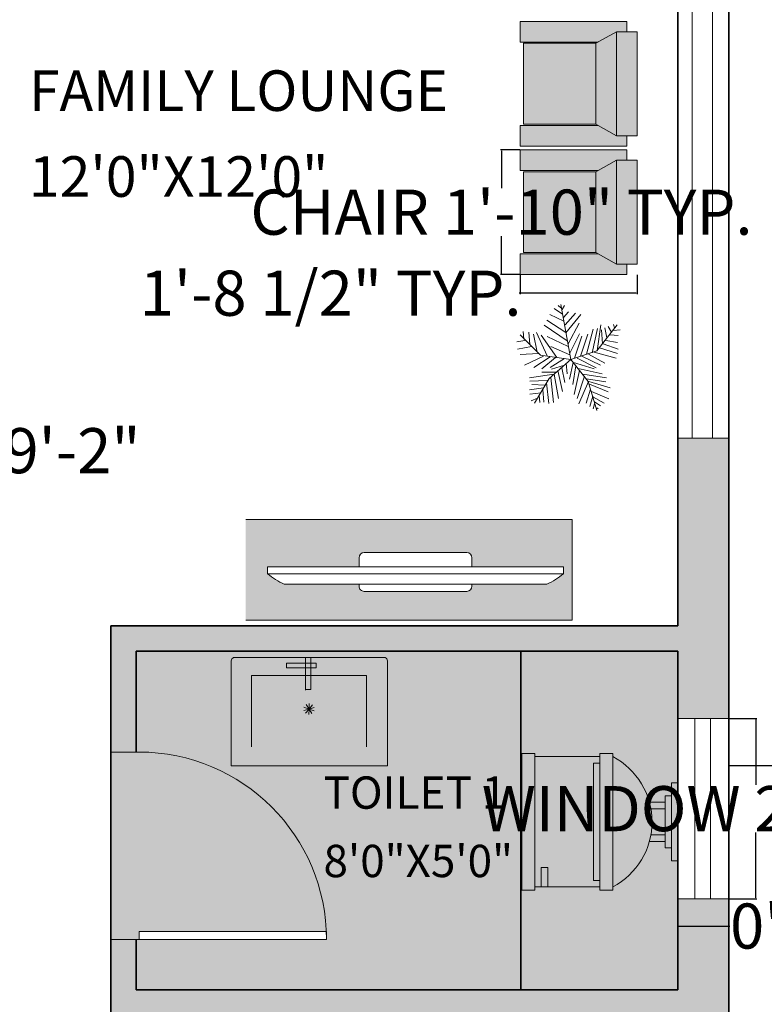
# Model space of a CAD drawing. Units: inches. Extents: x 853 to 1550, y 485 to 1596.
# Tile 10 of 18: x 1288 to 1420, y 1034 to 1208. Entities that reach past the tile are written whole.
import ezdxf

# ---------------------------------------------------------------- set-up
doc = ezdxf.new("R2010")
doc.units = ezdxf.units.IN
doc.header["$MEASUREMENT"] = 0
for name, color, linetype, lineweight in [('A-ANNO-DIMS', 2, 'Continuous', 18), ('A-AREA-IDEN', 250, 'Continuous', 18), ('A-DOOR', 4, 'Continuous', 18), ('A-FLOR-CASE', 32, 'Continuous', 25), ('A-FLOR-FIXT', 8, 'Continuous', 18), ('A-WALL-PATT', 250, 'Continuous', 13), ('furniture', 250, 'Continuous', 18), ('L-PLNT-TREE', 106, 'Continuous', 13), ('walls', 250, 'Continuous', 35), ('windows', 4, 'Continuous', 18)]:
    doc.layers.add(name, color=color, linetype=linetype, lineweight=lineweight)
for name, color, linetype, lineweight, true_color in [('A-FIXT-PATT', 9, 'Continuous', 13, 0xc7c8ca), ('A-FLOR-TILE-PATT', 141, 'Continuous', 13, 0xadddf7), ('A-FURN-PATT', 254, 'Continuous', 13, 0xfeeab9)]:
    doc.layers.add(name, color=color, linetype=linetype, lineweight=lineweight, true_color=true_color)
doc.styles.get("Standard").update_dxf_attribs({"font": 'arial.ttf'})
doc.dimstyles.get("Standard").update_dxf_attribs({"dimtxt": 8, "dimasz": 0.18, "dimexe": 0.18, "dimexo": 0.0625, "dimgap": 0.09, "dimtad": 0, "dimtih": 1, "dimtoh": 1, "dimzin": 0, "dimdsep": 46, "dimlunit": 3, "dimtxsty": 'Standard', "dimcen": 0.09, "dimadec": 0, "dimazin": 0, "dimtfac": 1, "dimtofl": 0, "dimtmove": 0, "dimatfit": 3, "dimfxl": 1, "dimtolj": 1, "dimtzin": 0, "dimarcsym": 0})

# ---------------------------------------------------------------- blocks, each defined once
blk = doc.blocks.new('*U10')
for p, q in [((0, 0), (0, -6)), ((40, 0), (40, -6))]:
    blk.add_line(p, q)
blk.add_lwpolyline([(0, 0), (0, 40), (1.75, 40), (1.75, 0)], close=True)
blk.add_arc((0, 0), 40, 0, 90)
blk = doc.blocks.new('FABRIC SOFA 1S')
at = {"layer": 'furniture'}
for p, q in [((3, 18.12), (34, 18.12)), ((3, 15.12), (3, 18.12)), ((34, 12.12), (34, 18.12)), ((0, -15.12), (0, 15.12)), ((6, 15.12), (0, 15.12)), ((6, -15.12), (6, 15.12)), ((12, 11.75), (6, 15.12)), ((11.33, 12.12), (34, 12.12)), ((6, -15.12), (12, -11.75)), ((11.33, -12.12), (34, -12.12)), ((34, -12.12), (34, -18.12)), ((6, -15.12), (0, -15.12)), ((3, -18.12), (3, -15.12)), ((3, -18.12), (34, -18.12))]:
    blk.add_line(p, q, dxfattribs=at)
blk.add_lwpolyline([(12, -11.75), (12, 11.75), (33, 11.75), (33, -11.75)], close=True, dxfattribs=at)
blk = doc.blocks.new('*U5')
for p, q in [((-10, 22), (-10, 12)), ((10, 12), (10, 22)), ((-10, 21), (-7, 21)), ((-7, 20), (-10, 20)), ((-7, 21), (-7, 20)), ((9, 13), (-9, 13)), ((-9, 13), (-9, 12)), ((9, 12), (9, 13)), ((10.5, 12), (-10.5, 12)), ((-10.5, 10), (-10.5, 12)), ((10.5, 12), (10.5, 10)), ((10.5, 10), (-10.5, 10)), ((-3, 4.4065), (-3, 2)), ((-2, 2), (-2, 4.1658)), ((2, 4.1658), (2, 2)), ((3, 2), (3, 4.4065)), ((4, 2), (-4, 2)), ((-4, 2), (-4, 1)), ((4, 1), (4, 2))]:
    blk.add_line(p, q)
for points in [[(10.5, 22), (10.5, 24), (-10.5, 24), (-10.5, 22)], [(6, 0), (6, 1), (-6, 1), (-6, 0)]]:
    blk.add_lwpolyline(points, close=True)
blk.add_arc((0, 15.3333), 11.3333, 208.0725, 331.9275)
blk = doc.blocks.new('*D20')
at = {"layer": 'A-ANNO-DIMS', "color": 0, "lineweight": -2, "transparency": 16777216}
for p, q in [((1413.94, 1090.29), (1413.94, 1075.73)), ((1437.94, 1090.29), (1437.94, 1075.73)), ((1414.12, 1075.91), (1422.1, 1075.91)), ((1437.76, 1075.91), (1429.78, 1075.91))]:
    blk.add_line(p, q, dxfattribs=at)
at = {"layer": 'A-ANNO-DIMS', "color": 0, "transparency": 16777216}
for points in [[(1414.12, 1075.94), (1414.12, 1075.88), (1413.94, 1075.91)], [(1437.76, 1075.94), (1437.76, 1075.88), (1437.94, 1075.91)]]:
    blk.add_solid(points, dxfattribs=at)
at = {"layer": 'Defpoints', "color": 0, "transparency": 16777216}
for p in [(1413.94, 1090.36), (1437.94, 1090.36), (1437.94, 1075.91)]:
    blk.add_point(p, dxfattribs=at)
at = {"layer": 'A-ANNO-DIMS', "color": 0, "transparency": 16777216, "insert": (1425.94, 1075.91), "char_height": 8, "attachment_point": 5}
blk.add_mtext("\\A1;2'", dxfattribs=at)
blk = doc.blocks.new('*U18')
for p, q in [((-8.737, 47.138), (-17.069, 52.711)), ((-10.186, 53.64), (-13.084, 55.962)), ((0, 0), (-10.5, 57)), ((-9.099, 51.782), (-6.563, 55.962)), ((-7.288, 39.707), (-21.778, 46.673)), ((-7.65, 43.423), (-2.578, 49.46)), ((-5.839, 35.992), (4.667, 48.067)), ((-5.114, 27.632), (10.463, 46.673)), ((-3.665, 19.273), (-27.574, 35.527)), ((-5.114, 28.097), (-24.676, 40.636)), ((-2.941, 16.486), (8.652, 37.85)), ((16.259, 5.805), (23.142, 31.348)), ((22.055, 7.198), (27.489, 32.277)), ((27, 9), (48, 36)), ((27.127, 9.056), (31.112, 35.992)), ((31.836, 30.883), (32.561, 16.486)), ((35.096, 32.741), (37.27, 22.524)), ((38.719, 34.134), (41.979, 28.561)), ((43.791, 29.954), (51.036, 30.883)), ((44.153, 36.456), (45.239, 32.741)), ((-31.5, 4.5), (-52.5, 25.5)), ((-48.585, 21.131), (-49.309, 29.026)), ((-43.513, 28.561), (-42.427, 15.558)), ((-38.442, 26.239), (-34.819, 7.663)), ((-35.544, 28.097), (-24.314, 3.947)), ((-14.533, 2.09), (-30.834, 25.31)), ((-24.314, 23.917), (-2.941, 13.7)), ((-1.129, 6.734), (9.014, 26.704)), ((3.942, 1.625), (11.187, 24.381)), ((10.101, 3.483), (17.708, 26.239)), ((40.53, 25.775), (48.862, 24.846)), ((-47.498, 19.737), (-55.83, 18.344)), ((-40.615, 13.7), (-55.105, 10.913)), ((-20.691, 13.7), (-1.129, 4.876)), ((29.662, 12.307), (48.137, 6.269)), ((33.285, 16.486), (48.862, 10.913)), ((36.183, 19.737), (48.137, 17.88)), ((-33.37, 6.269), (-52.207, 5.34)), ((-28.299, 3.483), (-47.86, -5.805)), ((-21.416, 3.018), (-38.079, -8.128)), ((0, 0), (-31.5, 4.5)), ((-15.982, 2.09), (-30.11, -9.521)), ((0, 0), (-22.5, -19.5)), ((-6.563, 1.161), (-21.416, -8.128)), ((0, 0), (27, 9)), ((0, 0), (18, -22.5)), ((6.478, 1.625), (26.04, -8.592)), ((11.187, 3.483), (30.749, -5.805)), ((18.07, 5.805), (35.096, -3.483)), ((24.229, 7.663), (46.688, 1.625)), ((-6.563, -5.805), (-19.967, -9.985)), ((-9.461, -8.592), (-6.201, -23.453)), ((-4.752, -3.483), (-3.665, -14.629)), ((2.493, -3.019), (-1.491, -20.202)), ((1.769, -2.555), (24.229, -9.521)), ((5.029, -6.27), (2.131, -25.775)), ((7.565, -9.056), (32.198, -14.629)), ((-17.431, -15.094), (-42.789, -18.809)), ((-22.5, -19.5), (-37.5, -45)), ((-15.257, -12.772), (-30.11, -12.772)), ((-20.691, -18.345), (-17.793, -44.352)), ((-17.069, -15.094), (-12.721, -40.172)), ((-13.446, -11.378), (-8.737, -32.741)), ((9.014, -11.378), (3.58, -35.992)), ((14.085, -16.951), (6.478, -40.172)), ((12.274, -15.094), (36.907, -18.809)), ((16.259, -19.738), (36.183, -22.989)), ((-28.299, -29.026), (-42.789, -31.348)), ((-24.314, -21.596), (-42.427, -22.06)), ((-26.849, -26.24), (-40.253, -25.775)), ((-25.038, -23.918), (-22.865, -45.281)), ((18.07, -22.524), (8.289, -45.745)), ((20.244, -30.419), (15.897, -44.816)), ((18, -22.5), (27, -52.5)), ((18.433, -22.524), (40.53, -29.026)), ((19.157, -25.311), (38.719, -33.206)), ((-30.834, -34.135), (-42.427, -35.528)), ((-34.457, -39.708), (-40.978, -42.494)), ((-32.646, -36.921), (-31.921, -44.352)), ((-29.023, -30.884), (-27.936, -43.887)), ((22.78, -37.85), (19.519, -48.532)), ((21.331, -32.741), (39.081, -40.636)), ((22.78, -38.314), (34.372, -44.816)), ((24.591, -45.745), (23.142, -50.854)), ((24.591, -43.423), (30.749, -47.603)), ((26.764, -49.925), (28.213, -50.854))]:
    blk.add_line(p, q)
blk = doc.blocks.new('BASIN-RECT-WITH-MIXER')
for p, q in [((0, 3.21), (0, 19.18)), ((0, 19.18), (27.7, 19.18)), ((27.7, 19.18), (27.7, 0.61)), ((3.57, 3.21), (3.57, 15.84)), ((24, 15.84), (24, 3.21)), ((13.79, 9.14), (12.86, 9.39)), ((13.79, 9.14), (12.89, 8.8)), ((13.79, 9.14), (13.18, 9.89)), ((13.79, 9.14), (13.26, 8.33)), ((13.79, 9.14), (13.74, 10.1)), ((13.79, 9.14), (14.31, 9.95)), ((13.79, 9.14), (14.69, 9.48)), ((13.79, 9.14), (14.39, 8.39)), ((13.79, 9.14), (13.83, 8.18)), ((13.79, 9.14), (14.72, 8.89)), ((13.18, 5.79), (13.18, 0)), ((14.12, 5.69), (13.18, 5.69)), ((14.12, 0), (14.12, 5.69)), ((0, 0.61), (0, 3.21)), ((24, 3.21), (3.57, 3.21)), ((15.05, 1.84), (9.82, 1.84)), ((9.82, 1.84), (9.82, 0.98)), ((15.05, 0.98), (15.05, 1.84)), ((27.28, 0), (0.42, 0)), ((9.82, 0.98), (11.8, 0.98)), ((11.8, 0.98), (15.05, 0.98))]:
    blk.add_line(p, q)
for centre, start, end in [((0.76, 0.68), 185.6886, 243.8456), ((26.94, 0.68), 296.1544, 354.3114)]:
    blk.add_arc(centre, 0.761, start, end)
blk = doc.blocks.new('WIN-BATH-32IN')
for p, q in [((0, 32.01), (9, 32.01)), ((0, 0), (0, 32.01)), ((0, 32.01), (3.01, 32.01)), ((3.01, 32.01), (3.01, 0)), ((5.76, 0), (5.76, 32.01)), ((9, 32.01), (9, 0)), ((9, 0), (0, 0)), ((3.01, 0), (5.76, 0))]:
    blk.add_line(p, q)
blk = doc.blocks.new('WIN-94IN')
for p, q in [((0, 94.25), (9, 94.25)), ((0, 0), (0, 94.25)), ((2.54, 94.25), (2.54, 0)), ((6.1, 0), (6.1, 94.25)), ((9, 94.25), (9, 0)), ((9, 0), (0, 0)), ((2.54, 0), (6.1, 0))]:
    blk.add_line(p, q)
blk = doc.blocks.new('PLASMA-LARGE')
at = {"layer": 'furniture'}
for p, q in [((-7.26, 0), (7.26, 0)), ((-18.61, -1), (18.61, -1)), ((-8, -1), (-8, -0.74)), ((8, -1), (8, -0.74)), ((-21, -2.5), (21, -2.5)), ((-21, -2.5), (-21, -3.5)), ((21, -2.5), (21, -3.5)), ((-21, -3.5), (21, -3.5)), ((-8, -3.5), (-8, -4.76)), ((8, -3.5), (8, -4.76)), ((-7.26, -5.5), (7.26, -5.5))]:
    blk.add_line(p, q, dxfattribs=at)
for centre, radius, start, end in [((-7.26, -0.74), 0.744, 90, 180), ((7.26, -0.74), 0.744, 0, 90), ((-13.97, -11.05), 11.07, 114.7602, 129.4175), ((13.97, -11.05), 11.07, 50.5825, 65.2398), ((-7.26, -4.76), 0.744, 180, 270), ((7.26, -4.76), 0.744, 270, 0)]:
    blk.add_arc(centre, radius, start, end, dxfattribs=at)
blk = doc.blocks.new('TV-CONSOLE')
for p, q in [((0, 0), (0, 57.83)), ((0, 57.83), (17.81, 57.83)), ((17.81, 57.83), (17.81, 0))]:
    blk.add_line(p, q)
at = {"xscale": 1.249763490704796, "yscale": 1.249763490704796, "zscale": 1.249763490704796, "rotation": 270}
blk.add_blockref('PLASMA-LARGE', (12.71, 30.08), dxfattribs=at)
blk = doc.blocks.new('*D35')
at = {"layer": 'A-ANNO-DIMS', "color": 0, "lineweight": -2, "transparency": 16777216}
for p, q in [((1376.91, 1184.98), (1373.48, 1184.98)), ((1373.66, 1184.8), (1373.66, 1178.17)), ((1373.66, 1163.07), (1373.66, 1169.71)), ((1376.91, 1162.89), (1373.48, 1162.89))]:
    blk.add_line(p, q, dxfattribs=at)
at = {"layer": 'A-ANNO-DIMS', "color": 0, "transparency": 16777216}
for points in [[(1373.63, 1184.8), (1373.69, 1184.8), (1373.66, 1184.98)], [(1373.63, 1163.07), (1373.69, 1163.07), (1373.66, 1162.89)]]:
    blk.add_solid(points, dxfattribs=at)
at = {"layer": 'Defpoints', "color": 0, "transparency": 16777216}
for p in [(1373.66, 1184.98), (1376.98, 1184.98), (1376.98, 1162.89)]:
    blk.add_point(p, dxfattribs=at)
at = {"layer": 'A-ANNO-DIMS', "color": 0, "transparency": 16777216, "insert": (1373.66, 1173.94), "char_height": 8, "attachment_point": 5}
blk.add_mtext('\\A1;CHAIR 1\'-10" TYP.', dxfattribs=at)
blk = doc.blocks.new('*D36')
at = {"layer": 'A-ANNO-DIMS', "color": 0, "lineweight": -2, "transparency": 16777216}
for p, q in [((1376.98, 1162.83), (1376.98, 1159.4)), ((1397.7, 1162.83), (1397.7, 1159.4)), ((1376.98, 1159.58), (1376.8, 1159.58)), ((1397.52, 1159.58), (1377.16, 1159.58))]:
    blk.add_line(p, q, dxfattribs=at)
at = {"layer": 'A-ANNO-DIMS', "color": 0, "transparency": 16777216}
for points in [[(1377.16, 1159.61), (1377.16, 1159.55), (1376.98, 1159.58)], [(1397.52, 1159.61), (1397.52, 1159.55), (1397.7, 1159.58)]]:
    blk.add_solid(points, dxfattribs=at)
at = {"layer": 'Defpoints', "color": 0, "transparency": 16777216}
for p in [(1376.98, 1162.89), (1397.7, 1162.89), (1376.98, 1159.58)]:
    blk.add_point(p, dxfattribs=at)
at = {"layer": 'A-ANNO-DIMS', "color": 0, "transparency": 16777216, "insert": (1343.38, 1159.58), "char_height": 8, "attachment_point": 5}
blk.add_mtext('\\A1;1\'-8 1/2" TYP.', dxfattribs=at)
blk = doc.blocks.new('*D53')
at = {"layer": 'A-ANNO-DIMS', "color": 0, "lineweight": -2, "transparency": 16777216}
for p, q in [((1414, 1084.23), (1418.92, 1084.23)), ((1418.74, 1084.05), (1418.74, 1072.46)), ((1418.74, 1052.41), (1418.74, 1064)), ((1414, 1052.23), (1418.92, 1052.23))]:
    blk.add_line(p, q, dxfattribs=at)
at = {"layer": 'A-ANNO-DIMS', "color": 0, "transparency": 16777216}
for points in [[(1418.71, 1084.05), (1418.77, 1084.05), (1418.74, 1084.23)], [(1418.71, 1052.41), (1418.77, 1052.41), (1418.74, 1052.23)]]:
    blk.add_solid(points, dxfattribs=at)
at = {"layer": 'Defpoints', "color": 0, "transparency": 16777216}
for p in [(1413.94, 1084.23), (1418.74, 1084.23), (1413.94, 1052.23)]:
    blk.add_point(p, dxfattribs=at)
at = {"layer": 'A-ANNO-DIMS', "color": 0, "transparency": 16777216, "insert": (1418.74, 1068.23), "char_height": 8, "attachment_point": 5}
blk.add_mtext('\\A1;WINDOW 2\'-8" TYP.', dxfattribs=at)
blk = doc.blocks.new('*D54')
at = {"layer": 'A-ANNO-DIMS', "color": 0, "lineweight": -2, "transparency": 16777216}
for p, q in [((1404.94, 1052.16), (1404.94, 1047.25)), ((1413.94, 1052.16), (1413.94, 1047.25)), ((1405.12, 1047.43), (1413.76, 1047.43)), ((1413.94, 1047.43), (1414.12, 1047.43))]:
    blk.add_line(p, q, dxfattribs=at)
at = {"layer": 'A-ANNO-DIMS', "color": 0, "transparency": 16777216}
for points in [[(1405.12, 1047.46), (1405.12, 1047.4), (1404.94, 1047.43)], [(1413.76, 1047.46), (1413.76, 1047.4), (1413.94, 1047.43)]]:
    blk.add_solid(points, dxfattribs=at)
at = {"layer": 'Defpoints', "color": 0, "transparency": 16777216}
for p in [(1404.94, 1052.23), (1413.94, 1052.23), (1413.94, 1047.43)]:
    blk.add_point(p, dxfattribs=at)
at = {"layer": 'A-ANNO-DIMS', "color": 0, "transparency": 16777216, "insert": (1438.59, 1047.43), "char_height": 8, "attachment_point": 5}
blk.add_mtext('\\A1;0\'-9" TYP.', dxfattribs=at)
blk = doc.blocks.new('*D67')
at = {"layer": 'A-ANNO-DIMS', "color": 0, "lineweight": -2, "transparency": 16777216}
for p, q in [((1250.4, 1186.71), (1267.03, 1186.71)), ((1266.85, 1186.53), (1266.85, 1135.89)), ((1266.85, 1076.81), (1266.85, 1127.44)), ((1250.4, 1076.63), (1267.03, 1076.63))]:
    blk.add_line(p, q, dxfattribs=at)
at = {"layer": 'A-ANNO-DIMS', "color": 0, "transparency": 16777216}
for points in [[(1266.82, 1186.53), (1266.88, 1186.53), (1266.85, 1186.71)], [(1266.82, 1076.81), (1266.88, 1076.81), (1266.85, 1076.63)]]:
    blk.add_solid(points, dxfattribs=at)
at = {"layer": 'Defpoints', "color": 0, "transparency": 16777216}
for p in [(1250.34, 1186.71), (1266.85, 1186.71), (1250.34, 1076.63)]:
    blk.add_point(p, dxfattribs=at)
at = {"layer": 'A-ANNO-DIMS', "color": 0, "transparency": 16777216, "insert": (1266.85, 1131.67), "char_height": 8, "attachment_point": 5}
blk.add_mtext('\\A1;DINING SET 9\'-2"', dxfattribs=at)

msp = doc.modelspace()

# ---------------------------------------------------------------- hatches: boundary and pattern name
at = {"layer": 'A-FIXT-PATT'}
h = msp.add_hatch(color=256, dxfattribs=at)
h.dxf.hatch_style = 1
h.paths.add_polyline_path([(1349.763, 1079.188), (1329.326, 1079.188), (1329.326, 1091.817), (1338.94, 1091.817), (1338.94, 1089.338), (1339.876, 1089.338), (1339.876, 1091.817), (1349.763, 1091.817)])
h.paths.add_polyline_path([(1341.57, 1085.885, 1), (1337.519, 1085.885, 1)], flags=16)
h.paths.add_polyline_path([(1340.507, 1085.885, 1), (1338.582, 1085.885, 1)], flags=0)
h.paths.add_polyline_path([(1339.876, 1089.338), (1338.94, 1089.338), (1338.94, 1091.817), (1339.876, 1091.817)], flags=17)
h.paths.add_polyline_path([(1339.876, 1091.817), (1338.94, 1091.817), (1338.94, 1093.187), (1339.876, 1093.187)])
h.paths.add_polyline_path([(1339.876, 1093.187), (1338.94, 1093.187), (1338.94, 1094.047), (1339.876, 1094.047)])
h.paths.add_polyline_path([(1338.94, 1093.187), (1335.575, 1093.187), (1335.575, 1094.047), (1337.557, 1094.047), (1338.94, 1094.047)])
h.paths.add_polyline_path([(1340.811, 1093.187), (1339.876, 1093.187), (1339.876, 1094.047), (1340.811, 1094.047)])
h.paths.add_polyline_path([(1339.876, 1094.047), (1338.94, 1094.047), (1338.94, 1095.025), (1339.876, 1095.025)])
h.paths.add_polyline_path([(1339.876, 1095.025), (1338.94, 1095.025), (1338.94, 1096.137), (1339.876, 1096.137)])
h = msp.add_hatch(color=256, dxfattribs=at)
h.dxf.hatch_style = 1
h.paths.add_polyline_path([(1329.326, 1079.188), (1349.763, 1079.188), (1349.763, 1091.817), (1339.876, 1091.817), (1339.876, 1093.187), (1340.811, 1093.187), (1340.811, 1094.047), (1339.876, 1094.047), (1339.876, 1095.025), (1353.033, 1095.025, -0.2593488), (1353.455, 1094.417), (1353.455, 1075.844), (1325.759, 1075.844), (1325.759, 1091.817), (1325.759, 1094.417, -0.2593488), (1326.18, 1095.025), (1338.94, 1095.025), (1338.94, 1094.047), (1337.557, 1094.047), (1335.575, 1094.047), (1335.575, 1093.187), (1338.94, 1093.187), (1338.94, 1091.817), (1329.326, 1091.817)])
h = msp.add_hatch(color=256, dxfattribs=at)
h.dxf.hatch_style = 1
h.paths.add_polyline_path([(1337.519, 1085.885, -1), (1341.57, 1085.885, -1)])
h.paths.add_polyline_path([(1340.507, 1085.885, 1), (1338.582, 1085.885, 1)], flags=16)
h = msp.add_hatch(color=256, dxfattribs=at)
h.dxf.hatch_style = 1
h.paths.add_polyline_path([(1379.551, 1077.46), (1379.551, 1054.359), (1380.706, 1054.359), (1380.706, 1057.824), (1381.861, 1057.824), (1381.861, 1054.359), (1391.102, 1054.359), (1391.102, 1055.514), (1389.947, 1055.514), (1389.947, 1076.305), (1391.102, 1076.305), (1391.102, 1077.46)])
h.paths.add_polyline_path([(1377.241, 1078.038), (1377.241, 1053.781), (1379.551, 1053.781), (1379.551, 1078.038)])
h.paths.add_polyline_path([(1391.102, 1078.038), (1391.102, 1053.781), (1393.412, 1053.781), (1393.412, 1078.038)])
h.paths.add_polyline_path([(1389.947, 1076.305), (1389.947, 1055.514), (1391.102, 1055.514), (1391.102, 1076.305)], flags=17)
h.paths.add_polyline_path([(1393.412, 1077.46), (1393.412, 1054.359, 0.6000022)])
h.paths.add_polyline_path([(1400.137, 1063.599, -0.0226287), (1399.876, 1062.444), (1402.653, 1062.444), (1402.653, 1063.599)])
h.paths.add_polyline_path([(1399.876, 1069.375, -0.0226287), (1400.137, 1068.22), (1402.653, 1068.22), (1402.653, 1069.375)])
h.paths.add_polyline_path([(1402.653, 1070.53), (1402.653, 1061.289), (1403.808, 1061.289), (1403.808, 1070.53)])
h.paths.add_polyline_path([(1403.808, 1072.84), (1403.808, 1058.979), (1404.963, 1058.979), (1404.963, 1072.84)])
at = {"layer": 'A-FLOR-TILE-PATT'}
h = msp.add_hatch(dxfattribs=at)
h.set_pattern_fill('ANGLE', color=256)
h.set_pattern_definition([(0, (0, 0), (0, 0.275), [0.2, -0.075]), (90, (0, 0), (-0.275, 0), [0.2, -0.075])])
h.paths.add_polyline_path([(1309.421, 1078.26), (1304.437, 1078.26), (1304.437, 1045.033), (1309.421, 1045.033), (1309.421, 1046.486), (1342.617, 1046.486, 0.4014527)])
h.paths.add_polyline_path([(1377.065, 1096.129), (1308.937, 1096.129), (1308.937, 1078.26), (1309.421, 1078.26, -0.4014527), (1342.617, 1046.486), (1342.649, 1046.486), (1342.649, 1045.033), (1309.421, 1045.033), (1308.937, 1045.033), (1308.937, 1036.129), (1377.065, 1036.129)])
h.paths.add_polyline_path([(1404.937, 1096.129), (1377.065, 1096.129), (1377.065, 1036.129), (1404.937, 1036.129)])
at = {"layer": 'A-FURN-PATT'}
h = msp.add_hatch(color=256, dxfattribs=at)
h.dxf.hatch_style = 1
h.paths.add_polyline_path([(1390.384, 1203.865), (1377.586, 1203.865), (1377.586, 1189.543), (1390.384, 1189.543)])
h.paths.add_polyline_path([(1394.041, 1205.921), (1395.869, 1205.921), (1395.869, 1207.75), (1376.977, 1207.75), (1376.977, 1204.093), (1390.791, 1204.093)])
h.paths.add_polyline_path([(1394.041, 1205.921), (1390.384, 1203.865), (1390.384, 1189.543), (1394.041, 1187.486)])
h.paths.add_polyline_path([(1397.697, 1205.921), (1394.041, 1205.921), (1394.041, 1187.486), (1397.697, 1187.486)])
h.paths.add_polyline_path([(1390.791, 1189.315), (1376.977, 1189.315), (1376.977, 1185.658), (1395.869, 1185.658), (1395.869, 1187.486), (1394.041, 1187.486)])
h = msp.add_hatch(color=256, dxfattribs=at)
h.dxf.hatch_style = 1
h.paths.add_polyline_path([(1394.041, 1183.157), (1395.869, 1183.157), (1395.869, 1184.985), (1376.977, 1184.985), (1376.977, 1181.328), (1390.791, 1181.328)])
h.paths.add_polyline_path([(1394.041, 1183.157), (1390.384, 1181.1), (1390.384, 1166.778), (1394.041, 1164.721)])
h.paths.add_polyline_path([(1397.697, 1183.157), (1394.041, 1183.157), (1394.041, 1164.721), (1397.697, 1164.721)])
h.paths.add_polyline_path([(1395.869, 1164.721), (1394.041, 1164.721), (1390.791, 1166.55), (1376.977, 1166.55), (1376.977, 1162.893), (1395.869, 1162.893)])
h.paths.add_polyline_path([(1390.384, 1181.1), (1377.586, 1181.1), (1377.586, 1166.778), (1390.384, 1166.778)])
h = msp.add_hatch(color=256, dxfattribs=at)
h.dxf.hatch_style = 1
h.paths.add_polyline_path([(1386.179, 1119.452), (1328.345, 1119.452), (1328.345, 1101.641), (1386.179, 1101.641)])
h.paths.add_polyline_path([(1367.498, 1113.62, -0.4142136), (1368.428, 1112.689), (1368.428, 1111.12), (1384.675, 1111.12), (1384.675, 1109.87, -0.0640419), (1381.685, 1107.996), (1368.428, 1107.996), (1368.428, 1107.676, -0.4142136), (1367.498, 1106.746), (1349.362, 1106.746, -0.4142136), (1348.432, 1107.676), (1348.432, 1107.996), (1335.174, 1107.996, -0.0640419), (1332.185, 1109.87), (1332.185, 1111.12), (1348.432, 1111.12), (1348.432, 1112.689, -0.4142136), (1349.362, 1113.62)], flags=16)
at = {"layer": 'A-WALL-PATT'}
h = msp.add_hatch(color=256, dxfattribs=at)
h.dxf.hatch_style = 1
h.paths.add_polyline_path([(1139.437, 988.732), (1134.937, 988.732), (1134.937, 830.473), (1139.437, 830.473)])
h.paths.add_polyline_path([(1413.937, 1052.227), (1404.937, 1052.227), (1404.937, 1036.129), (1308.937, 1036.129), (1308.937, 1045.033), (1304.437, 1045.033), (1304.437, 1030.033), (1308.937, 1030.033), (1308.937, 1031.629), (1404.937, 1031.629), (1404.937, 863.629), (1365.241, 863.629), (1365.241, 854.629), (1413.937, 854.629)])
h.paths.add_polyline_path([(1413.937, 1133.918), (1404.937, 1133.918), (1404.937, 1100.629), (1304.437, 1100.629), (1304.437, 1078.26), (1308.937, 1078.26), (1308.937, 1096.129), (1404.937, 1096.129), (1404.937, 1084.233), (1407.946, 1084.233), (1413.937, 1084.233)])
h.paths.add_polyline_path([(1268.437, 1417.129), (1288.974, 1417.129), (1288.974, 1426.129), (1244.597, 1426.129), (1244.597, 1417.129), (1263.937, 1417.129), (1263.937, 1321.129), (1260.34, 1321.129), (1260.34, 1316.629), (1263.937, 1316.629), (1263.937, 1283.505), (1268.437, 1283.505)])
h.paths.add_polyline_path([(1413.937, 1426.129), (1360.402, 1426.129), (1360.402, 1417.129), (1404.937, 1417.129), (1404.937, 1249.129), (1268.437, 1249.129), (1268.437, 1254.041), (1268.357, 1254.041), (1263.937, 1254.041), (1263.937, 1244.629), (1404.937, 1244.629), (1404.937, 1228.163), (1413.937, 1228.163)])
h.paths.add_polyline_path([(1215.842, 1426.129), (1184.201, 1426.129), (1184.201, 1417.129), (1199.437, 1417.129), (1199.437, 1321.129), (1172.101, 1321.129), (1172.101, 1316.629), (1229.433, 1316.629), (1229.433, 1321.129), (1203.937, 1321.129), (1203.937, 1417.129), (1215.842, 1417.129)])
h.paths.add_polyline_path([(1139.437, 1417.129), (1155.446, 1417.129), (1155.446, 1426.129), (1091.831, 1426.129), (1091.831, 1417.129), (1134.937, 1417.129), (1134.937, 1289.22), (1139.437, 1289.22), (1139.437, 1316.629), (1143.553, 1316.629), (1143.553, 1321.129), (1139.437, 1321.129)])
h.paths.add_polyline_path([(1139.437, 1255.161), (1134.937, 1255.161), (1134.937, 1249.129), (990.937, 1249.129), (990.937, 1417.129), (1020.402, 1417.129), (1020.402, 1426.129), (981.937, 1426.129), (981.937, 1205.535), (984.477, 1205.535), (990.937, 1205.535), (990.937, 1244.629), (1134.937, 1244.629), (1134.937, 1237.775), (1139.437, 1237.775)])

# ---------------------------------------------------------------- linework, layer by layer
at = {"layer": 'A-FLOR-CASE'}
for p, q in [((1377.065, 1096.129), (1377.065, 1036.129)), ((1377.065, 1036.103), (1377.065, 1096.103))]:
    msp.add_line(p, q, dxfattribs=at)
at = {"layer": 'walls'}
for p, q in [((1413.937, 1426.129), (1413.937, 854.629)), ((1404.937, 1244.629), (1404.937, 1100.629)), ((1304.437, 1100.629), (1404.937, 1100.629)), ((1304.437, 1100.629), (1304.437, 989.436)), ((1308.937, 1096.129), (1404.937, 1096.129)), ((1308.937, 1096.129), (1308.937, 1078.26)), ((1404.937, 1096.129), (1404.937, 1036.129)), ((1308.937, 1045.033), (1308.937, 1036.129)), ((1308.937, 1036.129), (1404.937, 1036.129))]:
    msp.add_line(p, q, dxfattribs=at)

# ---------------------------------------------------------------- block references
at = {"layer": 'A-DOOR', "xscale": -0.8306897446249223, "yscale": 0.8306897446249223, "zscale": 0.8306897446249223, "rotation": 270}
msp.add_blockref('*U10', (1309.421, 1045.033), dxfattribs=at)
at = {"layer": 'A-FLOR-FIXT', "extrusion": (0, 0, -1), "zscale": -1, "rotation": 180}
msp.add_blockref('BASIN-RECT-WITH-MIXER', (-1325.758, 1095.025), dxfattribs=at)
at = {"layer": 'A-FLOR-FIXT', "xscale": 1.155096372646877, "yscale": 1.155096372646877, "zscale": 1.155096372646877, "rotation": 90.00000000000003}
msp.add_blockref('*U5', (1404.963, 1065.909), dxfattribs=at)
at = {"layer": 'furniture', "xscale": -0.6094251026746103, "yscale": 0.6094251026746103, "zscale": 0.6094251026746103}
for p in [(1397.697, 1196.704), (1397.697, 1173.939)]:
    msp.add_blockref('FABRIC SOFA 1S', p, dxfattribs=at)
at = {"layer": 'furniture', "rotation": 270.0000000000017}
msp.add_blockref('TV-CONSOLE', (1328.345, 1119.453), dxfattribs=at)
at = {"layer": 'L-PLNT-TREE', "xscale": 0.1715204275191126, "yscale": 0.1715204275191126, "zscale": 0.1715204275191126}
msp.add_blockref('*U18', (1385.955, 1147.804), dxfattribs=at)
at = {"layer": 'windows'}
for name, p in [('WIN-94IN', (1404.937, 1133.918)), ('WIN-BATH-32IN', (1404.937, 1052.226))]:
    msp.add_blockref(name, p, dxfattribs=at)

# ---------------------------------------------------------------- texts
at = {"layer": 'A-AREA-IDEN'}
for s, height, p in [('FAMILY LOUNGE', 7.19435, (1289.909, 1191.877)), ('12\'0"X12\'0"', 7.19435, (1289.909, 1176.658)), ('TOILET 1', 5.729, (1342.115, 1068.215)), ('8\'0"X5\'0"', 5.729, (1342.115, 1056.096))]:
    msp.add_text(s, height=height, dxfattribs=at).set_placement(p)

# ---------------------------------------------------------------- dimensions: what is measured, and where the dimension line sits
at = {"layer": 'A-ANNO-DIMS'}
for base, p1, p2, angle, text, picture, middle in [((1373.663, 1184.985), (1376.977, 1162.893), (1376.977, 1184.985), 90, 'CHAIR <> TYP.', '*D35', (1373.663, 1173.939)), ((1266.852, 1186.706), (1250.34, 1076.629), (1250.34, 1186.706), 90, 'DINING SET <>', '*D67', (1266.852, 1131.668)), ((1376.977, 1159.579), (1397.697, 1162.893), (1376.977, 1162.893), 180, '<> TYP.', '*D36', (1343.381, 1159.579)), ((1418.738, 1084.233), (1413.937, 1052.227), (1413.937, 1084.233), 90, 'WINDOW <> TYP.', '*D53', (1418.738, 1068.23))]:
    dim = msp.add_linear_dim(base=base, p1=p1, p2=p2, angle=angle, text=text, dimstyle='Standard', override={"dimdec": 1, "dimlfac": 1, "dimrnd": 0, "dimzin": 1, "dimdsep": 46, "dimlunit": 4, "dimfrac": 2}, dxfattribs=at)
    dim.commit()
    dim.dimension.update_dxf_attribs({"geometry": picture, "text_midpoint": middle})
dim = msp.add_linear_dim(base=(1437.937, 1075.913), p1=(1413.937, 1090.357), p2=(1437.937, 1090.357), dimstyle='Standard', override={"dimclrd": 0, "dimclre": 0, "dimclrt": 0}, dxfattribs=at)
dim.commit()
dim.dimension.update_dxf_attribs({"geometry": '*D20', "text_midpoint": (1425.937, 1075.913)})
dim = msp.add_linear_dim(base=(1413.937, 1047.426), p1=(1404.937, 1052.227), p2=(1413.937, 1052.227), text='<> TYP.', dimstyle='Standard', override={"dimdec": 1, "dimlfac": 1, "dimrnd": 0, "dimzin": 1, "dimdsep": 46, "dimlunit": 4, "dimfrac": 2}, dxfattribs=at)
dim.commit()
dim.dimension.update_dxf_attribs({"geometry": '*D54', "text_midpoint": (1438.589, 1047.426)})

doc.saveas('drawing.dxf')
